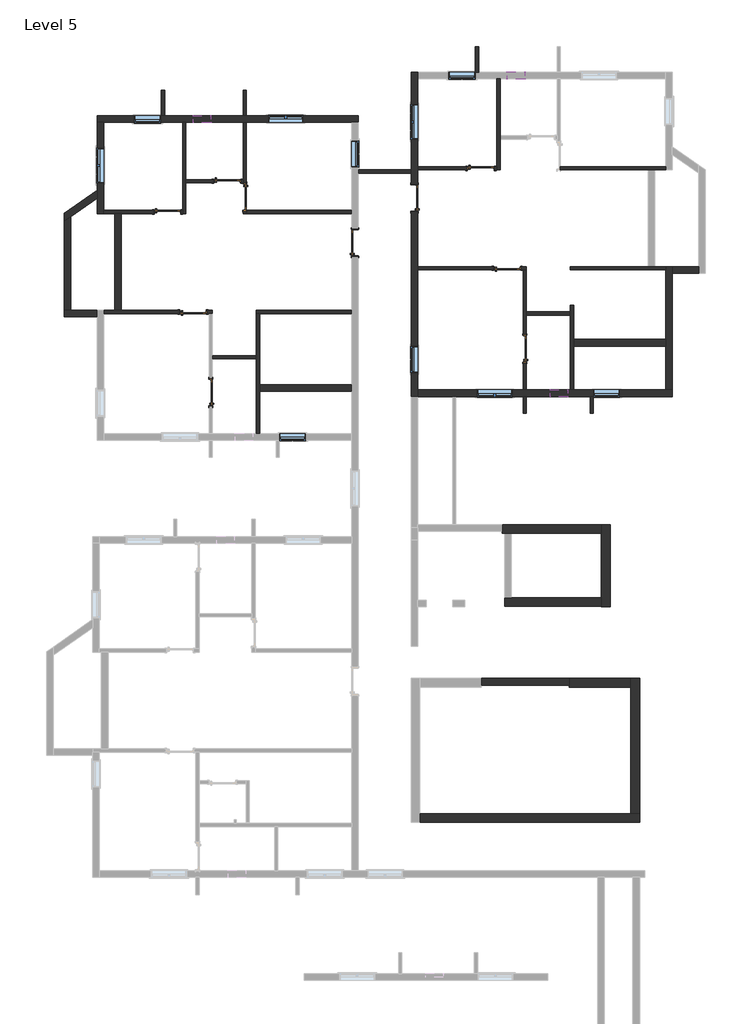
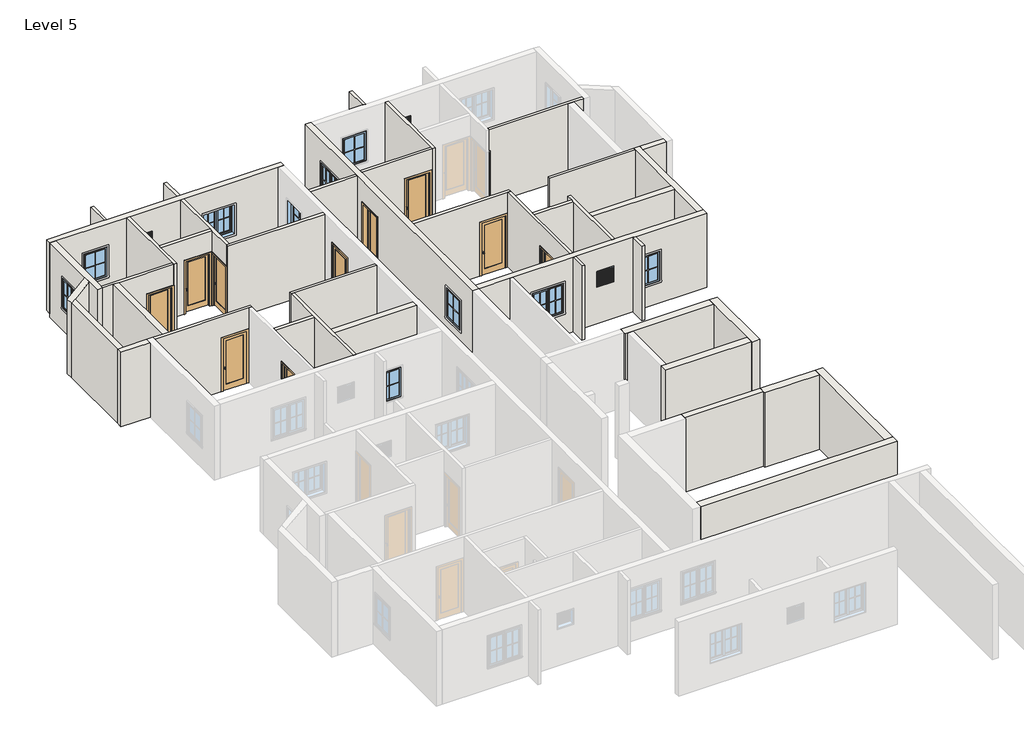
# One storey, part 5 of 7: 42 walls, 13 windows, 10 doors.
# Revit data of these elements (continued)
# Element 54 (IfcWindow, "Window-Awning-Single : 36\" x 48\"") (continued)
#   Interior Wall Closure = 0' - 2 1/4"
#   Frame Extension = 0' - 0 1/4"
#   Exterior Wall Closure = 0' - 1 1/4"
#   Interior Trim Visibility = yes
#   Exterior Trim Visibility = yes
#   Phase Created = New Construction
#   Materials on its faces: "Wood - Stained", "Glass", "Clad - White"
# Element 55 (IfcWindow, "Window-Awning-Single : 36\" x 48\"")
#   Mark = "86"
#   Window Inset = 0' - 0"
#   Interior Wall Closure = 0' - 2 1/4"
#   Frame Extension = 0' - 0 1/4"
#   Exterior Wall Closure = 0' - 1 1/4"
#   Interior Trim Visibility = yes
#   Exterior Trim Visibility = yes
#   Phase Created = New Construction
#   Materials on its faces: "Wood - Stained", "Glass", "Clad - White"
# Element 56 (IfcWindow, "Window-Awning-Single : 36\" x 48\"")
#   Mark = "88"
#   Window Inset = 0' - 0"
#   Interior Wall Closure = 0' - 2 1/4"
#   Frame Extension = 0' - 0 1/4"
#   Exterior Wall Closure = 0' - 1 1/4"
#   Interior Trim Visibility = yes
#   Exterior Trim Visibility = yes
#   Phase Created = New Construction
#   Materials on its faces: "Wood - Stained", "Glass", "Clad - White"
# Element 57 (IfcWindow, "Window-Awning-Single : 36\" x 48\"")
#   Mark = "90"
#   Window Inset = 0' - 0"
#   Interior Wall Closure = 0' - 2 1/4"
#   Frame Extension = 0' - 0 1/4"
#   Exterior Wall Closure = 0' - 1 1/4"
#   Interior Trim Visibility = yes
#   Exterior Trim Visibility = yes
#   Phase Created = New Construction
#   Materials on its faces: "Wood - Stained", "Glass", "Clad - White"
# Element 58 (IfcWindow, "Window-Awning-Single : 36\" x 48\"")
#   Mark = "91"
#   Window Inset = 0' - 0"
#   Interior Wall Closure = 0' - 2 1/4"
#   Frame Extension = 0' - 0 1/4"
#   Exterior Wall Closure = 0' - 1 1/4"
#   Interior Trim Visibility = yes
#   Exterior Trim Visibility = yes
#   Phase Created = New Construction
#   Materials on its faces: "Wood - Stained", "Glass", "Clad - White"
# Element 59 (IfcWindow, "Window-Casement-Double : 4' x 4'")
#   Mark = "100"
#   Window Inset = 0' - 0"
#   Interior Wall Closure = 0' - 2 1/4"
#   Frame Extension = 0' - 0 1/4"
#   Exterior Wall Closure = 0' - 1 1/4"
#   Interior Trim Visibility = yes
#   Exterior Trim Visibility = yes
#   Phase Created = New Construction
#   Materials on its faces: "Wood - Stained", "Glass", "Clad - White"
# Element 60 (IfcWindow, "Window-Casement-Double : 4' x 4'")
#   Mark = "101"
#   Window Inset = 0' - 0"
#   Interior Wall Closure = 0' - 2 1/4"
#   Frame Extension = 0' - 0 1/4"
#   Exterior Wall Closure = 0' - 1 1/4"
#   Interior Trim Visibility = yes
#   Exterior Trim Visibility = yes
#   Phase Created = New Construction
#   Materials on its faces: "Wood - Stained", "Glass", "Clad - White"
# Element 61 (IfcWindow, "Window-Casement-Double : 4' x 4'")
#   Mark = "103"
#   Window Inset = 0' - 0"
#   Interior Wall Closure = 0' - 2 1/4"
#   Frame Extension = 0' - 0 1/4"
#   Exterior Wall Closure = 0' - 1 1/4"
#   Interior Trim Visibility = yes
#   Exterior Trim Visibility = yes
#   Phase Created = New Construction
#   Materials on its faces: "Wood - Stained", "Glass", "Clad - White"
# Element 62 (IfcWindow, "Window-Casement-Double : 4' x 4'")
#   Mark = "105"
#   Window Inset = 0' - 0"
#   Interior Wall Closure = 0' - 2 1/4"
#   Frame Extension = 0' - 0 1/4"
#   Exterior Wall Closure = 0' - 1 1/4"
#   Interior Trim Visibility = yes
#   Exterior Trim Visibility = yes
#   Phase Created = New Construction
#   Materials on its faces: "Wood - Stained", "Glass", "Clad - White"
# Element 63 (IfcWindow, "Window-Louvers : 24\" x 24\"")
#   Mark = "67"
#   Blade Width = 1' - 10 1/2"
#   Phase Created = New Construction
#   Materials on its faces: "Birch"
# Element 64 (IfcWindow, "Window-Louvers : 24\" x 24\"")
#   Mark = "69"
#   Blade Width = 1' - 10 1/2"
#   Phase Created = New Construction
#   Materials on its faces: "Birch"
# Element 65 (IfcWindow, "Window-Louvers : 24\" x 24\"")
#   Mark = "70"
#   Blade Width = 1' - 10 1/2"
#   Phase Created = New Construction
#   Materials on its faces: "Birch"
# Materials
#   "Cherry": class "Wood", colour RGB 226 177 128, transparency 0, Description = "Prunus Serotina", Cost = 0
#   "Aluminum": class "Metal", colour RGB 247 247 247, transparency 0, Description = "Aluminum 6061", Cost = 0
#   "Wood - Stained": class "Wood", colour RGB 224 178 126, transparency 0, Cost = 0
#   "Glass": class "Glass", colour RGB 0 128 192, transparency 0.75, Description = "Soda Lime Glass", Cost = 0
#   "Clad - White": class "Wood", colour RGB 242 242 238, transparency 0, Cost = 0
#   "Birch": class "Wood", colour RGB 224 178 126, transparency 0, Description = "Betula Alleghaniensis", Cost = 0
#   "Default Wall": colour RGB 128 128 128, transparency 0, Cost = 0
